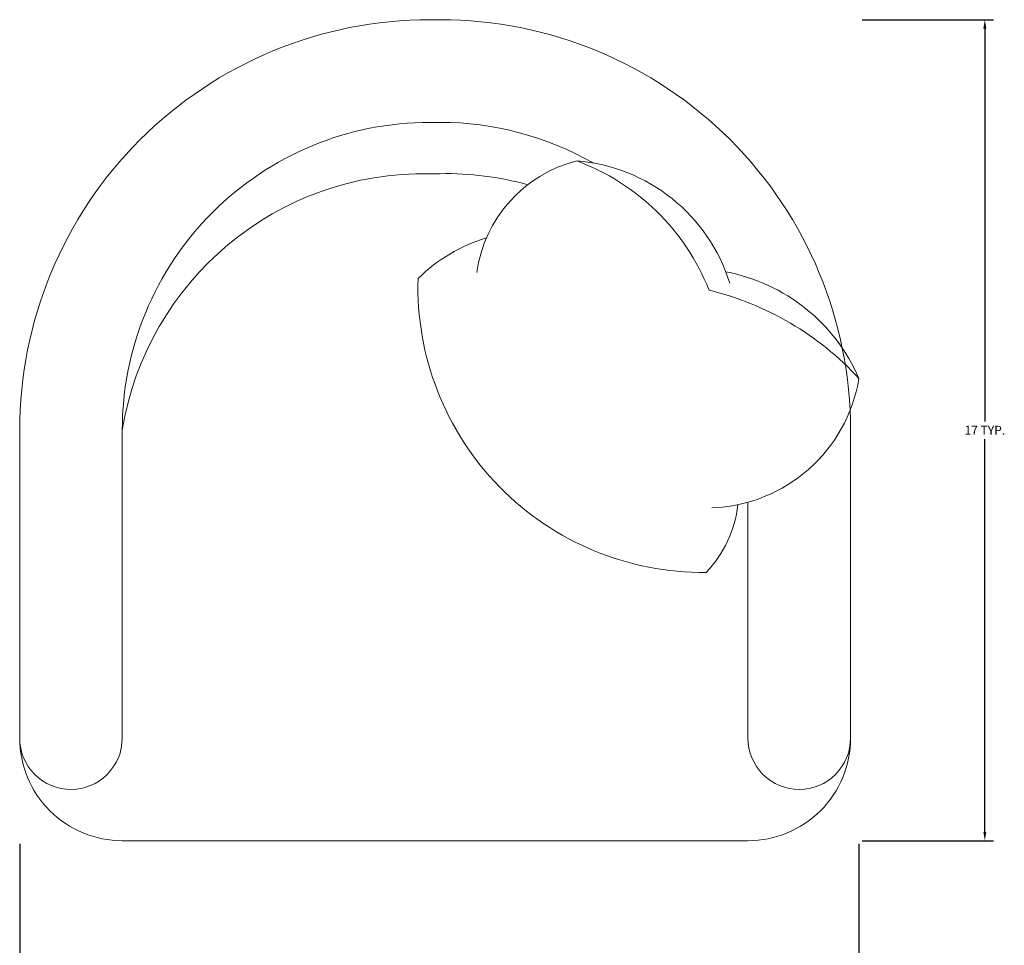
# Model space of a CAD drawing. Units: inches. Extents: x 963 to 2075, y 289 to 2657.
# Tile 25 of 98: x 1467.15 to 1487.2, y 1800.43 to 1819.27. Entities that reach past the tile are written whole.
import ezdxf

# ---------------------------------------------------------------- set-up
doc = ezdxf.new("R2010")
doc.units = ezdxf.units.IN
doc.layers.add('A-ANNO-DIMS', color=2, linetype='Continuous', lineweight=18)
doc.layers.add('A-FURN', color=8, linetype='Continuous', lineweight=18)
doc.styles.get("Standard").update_dxf_attribs({"font": 'arial.ttf'})
doc.dimstyles.get("Standard").update_dxf_attribs({"dimtxt": 0.18, "dimasz": 0.18, "dimexe": 0.18, "dimexo": 0.0625, "dimgap": 0.09, "dimtad": 0, "dimtih": 1, "dimtoh": 1, "dimdec": 4, "dimzin": 0, "dimdsep": 46, "dimtxsty": 'Standard', "dimcen": 0.09, "dimadec": 0, "dimazin": 0, "dimtfac": 1, "dimtdec": 4, "dimtofl": 0, "dimtmove": 0, "dimatfit": 3, "dimfxl": 1, "dimtolj": 1, "dimtzin": 0, "dimarcsym": 0})

# ---------------------------------------------------------------- blocks, each defined once
blk = doc.blocks.new('ARMCHAIR-C')
at = {"ltscale": 0.03}
blk.add_lwpolyline([(8.609, -0.446), (2.235, -0.446, -0.414214), (0.146, 1.643), (0.146, 7.912, -0.414214), (8.504, 16.271), (8.609, 16.271), (8.713, 16.271, -0.414214), (17.072, 7.912), (17.072, 1.643, -0.414214), (14.982, -0.446), (8.609, -0.446)], format="xyb", dxfattribs=at)
for points in [[(2.235, 7.912, -0.414214), (8.504, 14.181), (8.609, 14.181)], [(11.825, 13.354, 0.130591), (8.713, 14.181), (8.609, 14.181)], [(14.611, 10.906, 0.306663), (11.495, 13.396, 0.30633), (9.459, 11.122, -0.872847)], [(17.243, 8.967, 0.14773), (14.189, 10.763, 0.213343), (11.495, 13.396, 0.178662)], [(2.235, 7.912, -0.372719), (8.504, 13.136), (8.609, 13.136)], [(10.495, 12.911, 0.072384), (8.713, 13.136), (8.609, 13.136)], [(14.776, 6.397, -0.165541), (14.129, 5.017, -0.425989), (8.261, 11.002, -0.121523), (9.654, 11.827, 7.115464)], [(14.249, 6.333, 0.356772), (17.243, 8.967, 0.249542), (14.53, 11.137, -9.61688)], [(2.235, 7.912), (2.235, 1.643, -0.414214), (1.191, 0.598), (1.191, 0.598, -0.414214), (0.146, 1.643)], [(14.982, 6.447), (14.982, 1.643, 0.414214), (16.027, 0.598), (16.027, 0.598, 0.414214), (17.072, 1.643)]]:
    blk.add_lwpolyline(points, format="xyb")
blk = doc.blocks.new('*D26')
at = {"layer": 'A-ANNO-DIMS', "color": 0, "lineweight": -2, "transparency": 16777216}
for p, q in [((1467.146, 1802.491), (1467.146, 1799.809)), ((1484.243, 1802.491), (1484.243, 1799.809)), ((1467.326, 1799.989), (1474.33, 1799.989)), ((1484.063, 1799.989), (1477.059, 1799.989))]:
    blk.add_line(p, q, dxfattribs=at)
at = {"layer": 'A-ANNO-DIMS', "color": 0, "transparency": 16777216}
for points in [[(1467.326, 1800.019), (1467.326, 1799.959), (1467.146, 1799.989)], [(1484.063, 1800.019), (1484.063, 1799.959), (1484.243, 1799.989)]]:
    blk.add_solid(points, dxfattribs=at)
at = {"layer": 'Defpoints', "color": 0, "transparency": 16777216}
for p in [(1467.146, 1802.554), (1484.243, 1802.554), (1484.243, 1799.989)]:
    blk.add_point(p, dxfattribs=at)
at = {"layer": 'A-ANNO-DIMS', "color": 0, "transparency": 16777216, "insert": (1475.694, 1799.989), "char_height": 0.18, "attachment_point": 5}
blk.add_mtext('\\A1;ARMCHAIR C 17 TYP.', dxfattribs=at)
blk = doc.blocks.new('*D27')
at = {"layer": 'A-ANNO-DIMS', "color": 0, "lineweight": -2, "transparency": 16777216}
for p, q in [((1484.305, 1819.271), (1486.987, 1819.271)), ((1486.807, 1819.091), (1486.807, 1811.093)), ((1486.807, 1802.734), (1486.807, 1810.732)), ((1484.305, 1802.554), (1486.987, 1802.554))]:
    blk.add_line(p, q, dxfattribs=at)
at = {"layer": 'A-ANNO-DIMS', "color": 0, "transparency": 16777216}
for points in [[(1486.777, 1819.091), (1486.837, 1819.091), (1486.807, 1819.271)], [(1486.777, 1802.734), (1486.837, 1802.734), (1486.807, 1802.554)]]:
    blk.add_solid(points, dxfattribs=at)
at = {"layer": 'Defpoints', "color": 0, "transparency": 16777216}
for p in [(1484.243, 1819.271), (1486.807, 1819.271), (1484.243, 1802.554)]:
    blk.add_point(p, dxfattribs=at)
at = {"layer": 'A-ANNO-DIMS', "color": 0, "transparency": 16777216, "insert": (1486.807, 1810.912), "char_height": 0.18, "attachment_point": 5}
blk.add_mtext('\\A1;17 TYP.', dxfattribs=at)

msp = doc.modelspace()

# ---------------------------------------------------------------- block references
at = {"layer": 'A-FURN'}
msp.add_blockref('ARMCHAIR-C', (1467, 1803), dxfattribs=at)

# ---------------------------------------------------------------- dimensions: what is measured, and where the dimension line sits
at = {"layer": 'A-ANNO-DIMS'}
dim = msp.add_linear_dim(base=(1486.807, 1819.271), p1=(1484.243, 1802.554), p2=(1484.243, 1819.271), angle=90, text='<> TYP.', dimstyle='Standard', override={"dimdec": 0, "dimlfac": 1, "dimrnd": 0, "dimzin": 0, "dimdsep": 46, "dimlunit": 2}, dxfattribs=at)
dim.commit()
dim.dimension.update_dxf_attribs({"geometry": '*D27', "text_midpoint": (1486.807, 1810.912)})
dim = msp.add_linear_dim(base=(1484.243, 1799.989), p1=(1467.146, 1802.554), p2=(1484.243, 1802.554), text='ARMCHAIR C <> TYP.', dimstyle='Standard', override={"dimdec": 0, "dimlfac": 1, "dimrnd": 0, "dimzin": 0, "dimdsep": 46, "dimlunit": 2}, dxfattribs=at)
dim.commit()
dim.dimension.update_dxf_attribs({"geometry": '*D26', "text_midpoint": (1475.694, 1799.989)})

doc.saveas('drawing.dxf')
